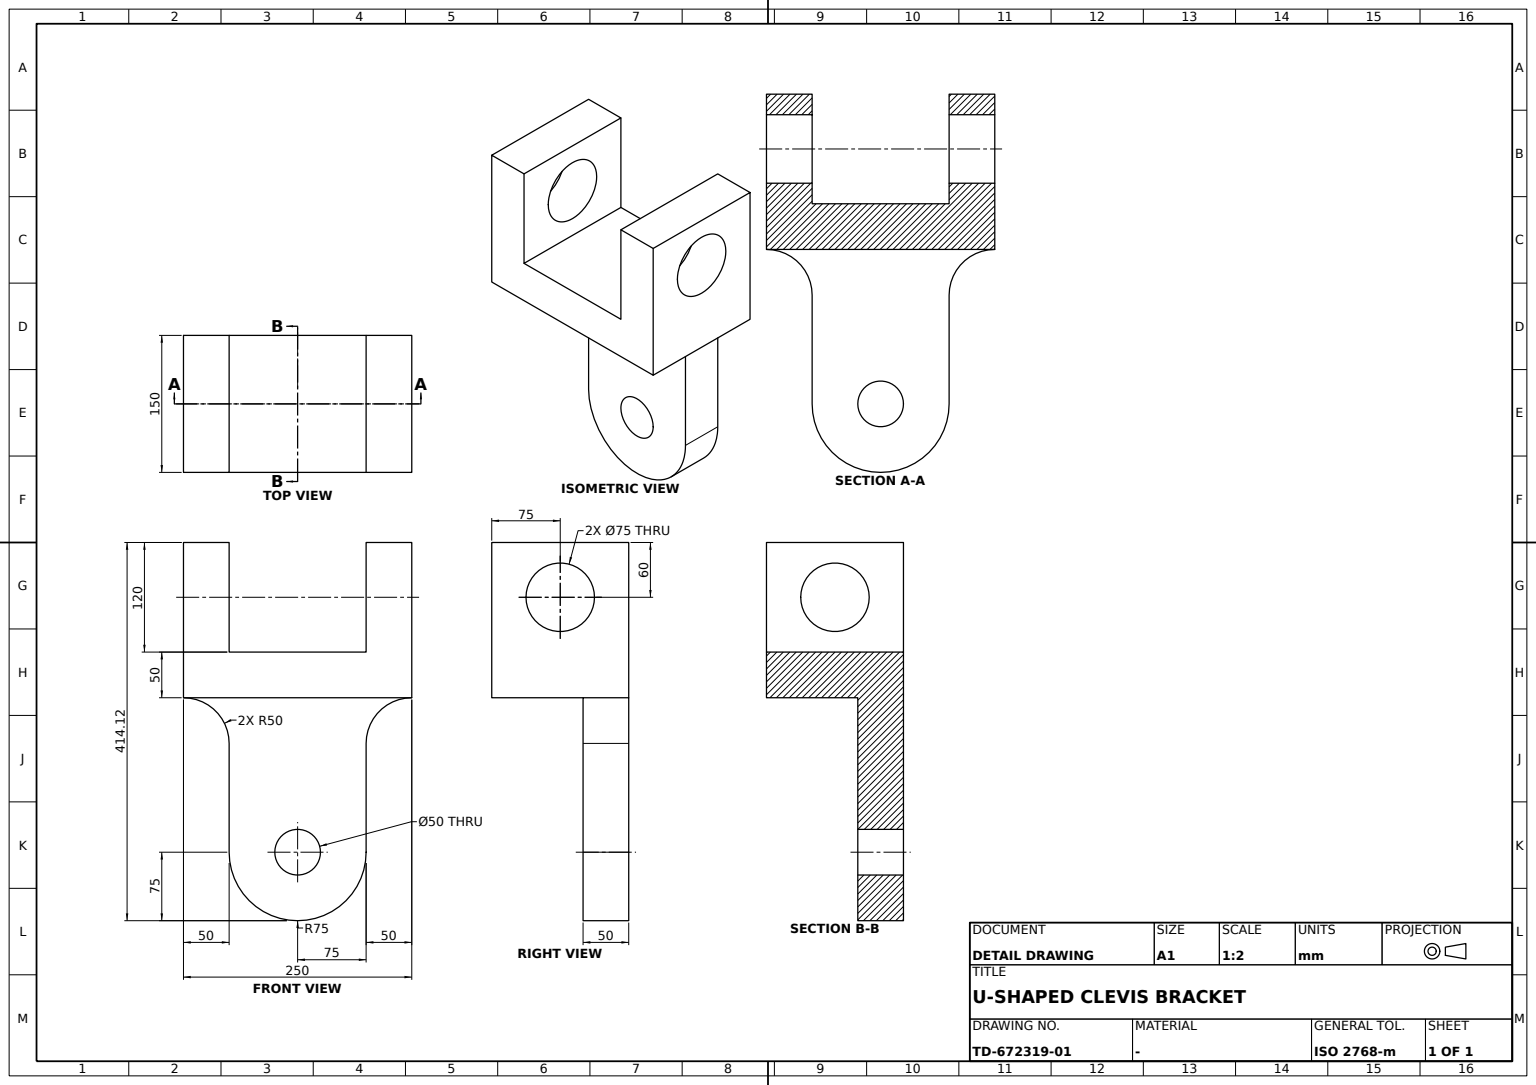
CATIA V5 part; units mm, degrees
sketch "Sketch1" plane through (0, 0, 0) normal (1, 0, 0) x (0, 1, 0)
  line L0 (-75, 0) -> (75, 0)
  point P0 (-75, 0)
  point P1 (75, 0)
  line L1 (75, 0) -> (75, 120)
  point P2 (75, 120)
  line L2 (75, 120) -> (125, 120)
  point P3 (125, 120)
  line L3 (125, 120) -> (125, -50)
  point P4 (125, -50)
  point P5 (-125, -50)
  point P6 (-125, 120)
  line L4 (-125, 120) -> (-125, -50)
  point P7 (-75, 120)
  point P8 (-75, 0)
  line L5 (-75, 0) -> (-75, 120)
  line L6 (-75, 120) -> (-125, 120)
  line L7 (-125, -50) -> (-125, -50)
  circle A0 centre (0, -219.1208) radius 25
  point P9 (0, -219.1208)
  arc A1 (-75, -219.1208) -> (75, -219.1208) centre (0, -219.1208) ccw
  point P10 (-75, -219.1208)
  line L8 (-75, -219.1208) -> (-75, -100)
  point P11 (75, -219.1208)
  line L9 (75, -219.1208) -> (75, -100)
  point P12 (75, -50)
  line L10 (125, -50) -> (125, -50)
  point P13 (-75, -219.1208)
  point P14 (75, -219.1208)
  arc A2 (-125, -50) -> (-75, -100) centre (-125, -100) cw
  arc A3 (125, -50) -> (75, -100) centre (125, -100) ccw
  line L11 (-125, -50) -> (125, -50) construction
  point P15 (125, -50)
  dimension "length L0" = 150
  dimension "radius A0" = 25
  dimension "radius A1" = 75
  dimension "distance L0 P9" = 219.1208
  dimension "radius A2" = 50
  dimension "radius A3" = 50
  dimension "distance P3 P4" = 170
  dimension "distance P2 P3" = 50
  dimension "distance P1 P2" = 120
  constraint midpoint L0 origin
  constraint horizontal L0 x-axis
  constraint horizontal L2 x-axis
  constraint horizontal L7 x-axis
  constraint horizontal L10 x-axis
  constraint vertical L1 y-axis
  constraint vertical L3 y-axis
  constraint vertical L8 y-axis
  constraint symmetry P4 P5 y-axis
  constraint symmetry P3 P6 y-axis
  constraint symmetry L3 L4 y-axis
  constraint symmetry P2 P7 y-axis
  constraint symmetry P1 P8 y-axis
  constraint symmetry L1 L5 y-axis
  constraint symmetry L2 L6 y-axis
  constraint coincidence P9 y-axis
  constraint coincidence P10 A1
  constraint coincidence P11 A1
  constraint coincidence P11 L1
  constraint coincidence P12 L7
  constraint coincidence L7 L10
  constraint coincidence L9 P14
  constraint coincidence L8 P13
  constraint coincidence L10 P12
  constraint coincidence L9 P12
  constraint coincidence P15 A3
  constraint coincidence P0 P8
  constraint coincidence P10 P13
  constraint coincidence P11 P14
  constraint tangency L9 A1
  constraint tangency L8 A1
  constraint tangency A2 L7
  constraint tangency A2 L8
  constraint tangency A3 L10
  constraint tangency A3 L9
  constraint tangency L11 A3
extrude "Pad1" add sketch "Sketch1" along normal mid plane 150
sketch "Sketch3" plane through (0, 125, 0) normal (0, 1, 0) x (-1, 0, 0)
  circle A0 centre (0, 60) radius 37.5
  point P0 (0, 60)
  line L0 (75, -50) -> (-75, -50) construction
  line L1 (75, -50) -> (75, 120) construction
  dimension "radius A0" = 37.5
  dimension "distance P0 L0" = 110
  dimension "distance P0 L1" = 75
extrude "Pocket1" cut sketch "Sketch3" against normal through all
sketch "Sketch4" plane through (0, -75, 0) normal (0, -1, 0) x (1, 0, 0)
  line L0 (-25, -50) -> (-25, -315.6473)
  line L1 (-25, -315.6473) -> (89.7281, -315.6473)
  line L2 (89.7281, -315.6473) -> (102.8052, -50)
  line L3 (102.8052, -50) -> (-25, -50)
  line L4 (-75, -100) -> (-75, -219.1208) construction
  line L5 (-75, -50) -> (75, -50) construction
  dimension "distance L4 L0" = 50
  constraint vertical L0 y-axis
  constraint horizontal L1 x-axis
  constraint horizontal L3 x-axis
  constraint coincidence L5 L3
extrude "Pocket2" cut sketch "Sketch4" along normal mid plane 500
sketch "Sketch2" plane through (-75, 0, 0) normal (-1, 0, 0) x (0, -1, 0)
properties part number "U-Shaped Mechanical Mounting Bracket with Circular Base Hole"
